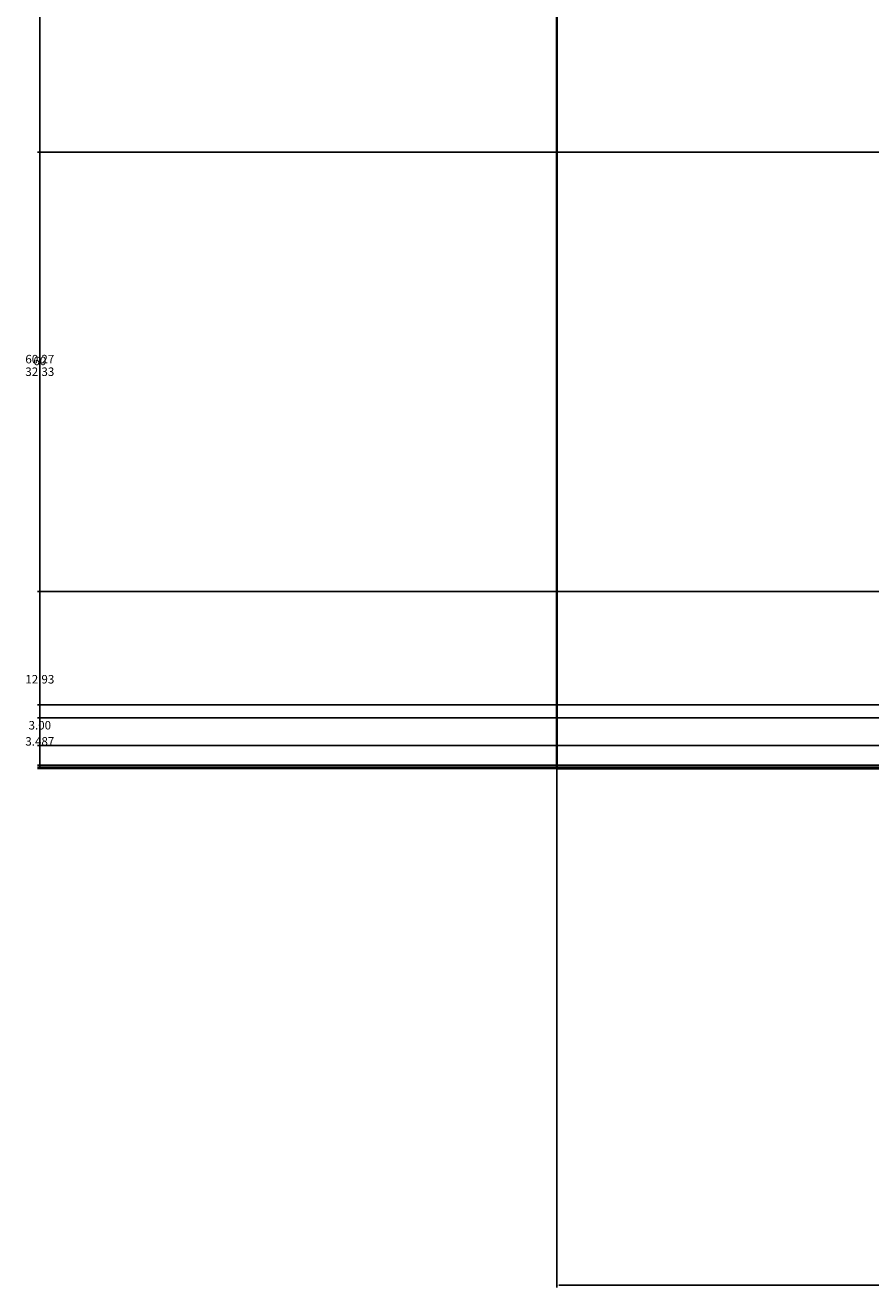
# Model space of a CAD drawing. Units: inches. Extents: x -13 to 809, y 112 to 656.
# Tile 1 of 55: x -13 to 49, y 112 to 205. Entities that reach past the tile are written whole.
import ezdxf

# ---------------------------------------------------------------- set-up
doc = ezdxf.new("R2010")
doc.units = ezdxf.units.IN
doc.header["$MEASUREMENT"] = 0
doc.layers.add('A-ANNO-DIMS', color=2, linetype='Continuous', lineweight=18)
doc.layers.add('A-ELEV', color=7, linetype='Continuous', lineweight=35)
doc.styles.get("Standard").update_dxf_attribs({"font": 'arial.ttf'})
doc.dimstyles.get("Standard").update_dxf_attribs({"dimtxt": 0.625, "dimasz": 0.18, "dimexe": 0.18, "dimexo": 0.0625, "dimgap": 0.09, "dimtad": 0, "dimtih": 1, "dimtoh": 1, "dimdec": 4, "dimzin": 0, "dimdsep": 46, "dimlunit": 4, "dimtxsty": 'Standard', "dimcen": 0.09, "dimadec": 0, "dimazin": 0, "dimtfac": 1, "dimtdec": 4, "dimtofl": 0, "dimtmove": 0, "dimatfit": 3, "dimfxl": 1, "dimtolj": 1, "dimtzin": 0, "dimarcsym": 0})

# ---------------------------------------------------------------- blocks, each defined once
blk = doc.blocks.new('*D11')
at = {"layer": 'A-ANNO-DIMS', "color": 0, "lineweight": -2, "transparency": 16777216}
for p, q in [((95.047, 306.457), (95.047, 112.34)), ((26.081, 150.457), (26.081, 112.34)), ((26.261, 112.52), (59.418, 112.52)), ((94.867, 112.52), (61.71, 112.52))]:
    blk.add_line(p, q, dxfattribs=at)
at = {"layer": 'A-ANNO-DIMS', "color": 0, "transparency": 16777216}
for points in [[(26.261, 112.55), (26.261, 112.49), (26.081, 112.52)], [(94.867, 112.55), (94.867, 112.49), (95.047, 112.52)]]:
    blk.add_solid(points, dxfattribs=at)
at = {"layer": 'Defpoints', "color": 0, "transparency": 16777216}
for p in [(95.047, 306.52), (26.081, 150.52), (95.047, 112.52)]:
    blk.add_point(p, dxfattribs=at)
at = {"layer": 'A-ANNO-DIMS', "color": 0, "transparency": 16777216, "insert": (60.564, 112.52), "char_height": 0.625, "attachment_point": 5}
blk.add_mtext('\\A1;68.97', dxfattribs=at)
blk = doc.blocks.new('*D32')
at = {"layer": 'A-ANNO-DIMS', "color": 0, "lineweight": -2, "transparency": 16777216}
for p, q in [((26.018, 210.52), (-12.099, 210.52)), ((-11.919, 210.34), (-11.919, 180.929)), ((-11.919, 150.7), (-11.919, 180.111)), ((26.018, 150.52), (-12.099, 150.52))]:
    blk.add_line(p, q, dxfattribs=at)
at = {"layer": 'A-ANNO-DIMS', "color": 0, "transparency": 16777216}
for points in [[(-11.949, 210.34), (-11.889, 210.34), (-11.919, 210.52)], [(-11.949, 150.7), (-11.889, 150.7), (-11.919, 150.52)]]:
    blk.add_solid(points, dxfattribs=at)
at = {"layer": 'Defpoints', "color": 0, "transparency": 16777216}
for p in [(-11.919, 210.52), (26.081, 210.52), (26.081, 150.52)]:
    blk.add_point(p, dxfattribs=at)
at = {"layer": 'A-ANNO-DIMS', "color": 0, "transparency": 16777216, "insert": (-11.919, 180.52), "char_height": 0.625, "attachment_point": 5}
blk.add_mtext('\\A1;60', dxfattribs=at)
blk = doc.blocks.new('*D90')
at = {"layer": 'A-ANNO-DIMS', "color": 0, "lineweight": -2, "transparency": 16777216}
for p, q in [((26.081, 210.457), (26.081, 112.34)), ((76.473, 195.828), (76.473, 112.34)), ((26.261, 112.52), (50.132, 112.52)), ((76.293, 112.52), (52.422, 112.52))]:
    blk.add_line(p, q, dxfattribs=at)
at = {"layer": 'A-ANNO-DIMS', "color": 0, "transparency": 16777216}
for points in [[(26.261, 112.55), (26.261, 112.49), (26.081, 112.52)], [(76.293, 112.55), (76.293, 112.49), (76.473, 112.52)]]:
    blk.add_solid(points, dxfattribs=at)
at = {"layer": 'Defpoints', "color": 0, "transparency": 16777216}
for p in [(26.081, 210.52), (76.473, 195.891), (76.473, 112.52)]:
    blk.add_point(p, dxfattribs=at)
at = {"layer": 'A-ANNO-DIMS', "color": 0, "transparency": 16777216, "insert": (51.277, 112.52), "char_height": 0.625, "attachment_point": 5}
blk.add_mtext('\\A1;50.39', dxfattribs=at)
blk = doc.blocks.new('*D91')
at = {"layer": 'A-ANNO-DIMS', "color": 0, "lineweight": -2, "transparency": 16777216}
for p, q in [((76.411, 163.564), (-12.099, 163.564)), ((-11.919, 163.384), (-11.919, 157.508)), ((-11.919, 150.814), (-11.919, 156.69)), ((77.515, 150.634), (-12.099, 150.634))]:
    blk.add_line(p, q, dxfattribs=at)
at = {"layer": 'A-ANNO-DIMS', "color": 0, "transparency": 16777216}
for points in [[(-11.949, 163.384), (-11.889, 163.384), (-11.919, 163.564)], [(-11.949, 150.814), (-11.889, 150.814), (-11.919, 150.634)]]:
    blk.add_solid(points, dxfattribs=at)
at = {"layer": 'Defpoints', "color": 0, "transparency": 16777216}
for p in [(-11.919, 163.564), (76.473, 163.564), (77.577, 150.634)]:
    blk.add_point(p, dxfattribs=at)
at = {"layer": 'A-ANNO-DIMS', "color": 0, "transparency": 16777216, "insert": (-11.919, 157.099), "char_height": 0.625, "attachment_point": 5}
blk.add_mtext('\\A1;12.93', dxfattribs=at)
blk = doc.blocks.new('*D92')
at = {"layer": 'A-ANNO-DIMS', "color": 0, "lineweight": -2, "transparency": 16777216}
for p, q in [((76.411, 195.891), (-12.099, 195.891)), ((-11.919, 195.711), (-11.919, 180.137)), ((-11.919, 163.744), (-11.919, 179.318)), ((76.411, 163.564), (-12.099, 163.564))]:
    blk.add_line(p, q, dxfattribs=at)
at = {"layer": 'A-ANNO-DIMS', "color": 0, "transparency": 16777216}
for points in [[(-11.949, 195.711), (-11.889, 195.711), (-11.919, 195.891)], [(-11.949, 163.744), (-11.889, 163.744), (-11.919, 163.564)]]:
    blk.add_solid(points, dxfattribs=at)
at = {"layer": 'Defpoints', "color": 0, "transparency": 16777216}
for p in [(-11.919, 195.891), (76.473, 195.891), (76.473, 163.564)]:
    blk.add_point(p, dxfattribs=at)
at = {"layer": 'A-ANNO-DIMS', "color": 0, "transparency": 16777216, "insert": (-11.919, 179.727), "char_height": 0.625, "attachment_point": 5}
blk.add_mtext('\\A1;32.33', dxfattribs=at)
blk = doc.blocks.new('*D115')
at = {"layer": 'A-ANNO-DIMS', "color": 0, "lineweight": -2, "transparency": 16777216}
for p, q in [((311.4, 210.785), (-12.099, 210.785)), ((-11.919, 210.605), (-11.919, 181.062)), ((-11.919, 150.7), (-11.919, 180.243)), ((311.637, 150.52), (-12.099, 150.52))]:
    blk.add_line(p, q, dxfattribs=at)
at = {"layer": 'A-ANNO-DIMS', "color": 0, "transparency": 16777216}
for points in [[(-11.949, 210.605), (-11.889, 210.605), (-11.919, 210.785)], [(-11.949, 150.7), (-11.889, 150.7), (-11.919, 150.52)]]:
    blk.add_solid(points, dxfattribs=at)
at = {"layer": 'Defpoints', "color": 0, "transparency": 16777216}
for p in [(-11.919, 210.785), (311.463, 210.785), (311.699, 150.52)]:
    blk.add_point(p, dxfattribs=at)
at = {"layer": 'A-ANNO-DIMS', "color": 0, "transparency": 16777216, "insert": (-11.919, 180.652), "char_height": 0.625, "attachment_point": 5}
blk.add_mtext('\\A1;60.27', dxfattribs=at)
blk = doc.blocks.new('*D117')
at = {"layer": 'A-ANNO-DIMS', "color": 0, "lineweight": -2, "transparency": 16777216}
for p, q in [((260.642, 154.272), (-12.099, 154.272)), ((-11.919, 154.092), (-11.919, 152.938)), ((-11.919, 150.965), (-11.919, 152.119)), ((258.04, 150.785), (-12.099, 150.785))]:
    blk.add_line(p, q, dxfattribs=at)
at = {"layer": 'A-ANNO-DIMS', "color": 0, "transparency": 16777216}
for points in [[(-11.949, 154.092), (-11.889, 154.092), (-11.919, 154.272)], [(-11.949, 150.965), (-11.889, 150.965), (-11.919, 150.785)]]:
    blk.add_solid(points, dxfattribs=at)
at = {"layer": 'Defpoints', "color": 0, "transparency": 16777216}
for p in [(260.705, 154.272), (-11.919, 150.785), (258.102, 150.785)]:
    blk.add_point(p, dxfattribs=at)
at = {"layer": 'A-ANNO-DIMS', "color": 0, "transparency": 16777216, "insert": (-11.919, 152.529), "char_height": 0.625, "attachment_point": 5}
blk.add_mtext('\\A1;3.487', dxfattribs=at)
blk = doc.blocks.new('*D131')
at = {"layer": 'A-ANNO-DIMS', "color": 0, "lineweight": -2, "transparency": 16777216}
for p, q in [((368.876, 155.214), (-12.099, 155.214)), ((-11.919, 155.034), (-11.919, 154.123)), ((-11.919, 152.394), (-11.919, 153.305)), ((365.876, 152.214), (-12.099, 152.214))]:
    blk.add_line(p, q, dxfattribs=at)
at = {"layer": 'A-ANNO-DIMS', "color": 0, "transparency": 16777216}
for points in [[(-11.949, 155.034), (-11.889, 155.034), (-11.919, 155.214)], [(-11.949, 152.394), (-11.889, 152.394), (-11.919, 152.214)]]:
    blk.add_solid(points, dxfattribs=at)
at = {"layer": 'Defpoints', "color": 0, "transparency": 16777216}
for p in [(368.938, 155.214), (-11.919, 152.214), (365.938, 152.214)]:
    blk.add_point(p, dxfattribs=at)
at = {"layer": 'A-ANNO-DIMS', "color": 0, "transparency": 16777216, "insert": (-11.919, 153.714), "char_height": 0.625, "attachment_point": 5}
blk.add_mtext('\\A1;3.00', dxfattribs=at)

msp = doc.modelspace()

# ---------------------------------------------------------------- linework, layer by layer
at = {"layer": 'A-ELEV'}
for p in [(26.0809, 210.5199), (109.5888, 150.5199)]:
    msp.add_line(p, (26.0809, 150.5199), dxfattribs=at)

# ---------------------------------------------------------------- dimensions: what is measured, and where the dimension line sits
at = {"layer": 'A-ANNO-DIMS'}
for base, p1, p2, picture, middle in [((95.0469, 112.5199), (26.0809, 150.5199), (95.0469, 306.5199), '*D11', (60.5639, 112.5199)), ((76.4733, 112.5199), (26.0809, 210.5199), (76.4733, 195.8907), '*D90', (51.2771, 112.5199))]:
    dim = msp.add_linear_dim(base=base, p1=p1, p2=p2, dimstyle='Standard', override={"dimdec": 2, "dimlfac": 1, "dimrnd": 0, "dimzin": 0, "dimdsep": 46, "dimlunit": 2}, dxfattribs=at)
    dim.commit()
    dim.dimension.update_dxf_attribs({"geometry": picture, "text_midpoint": middle})
for base, p1, p2, override, picture, middle in [((-11.91915, 210.78493), (311.6991, 150.51989), (311.46269, 210.78493), {"dimdec": 2, "dimlfac": 1, "dimrnd": 0, "dimzin": 0, "dimdsep": 46, "dimlunit": 2}, '*D115', (-11.91915, 180.65241)), ((-11.9191, 210.5199), (26.0809, 150.5199), (26.0809, 210.5199), {"dimdec": 0, "dimlfac": 1, "dimrnd": 0, "dimzin": 0, "dimdsep": 46, "dimlunit": 2}, '*D32', (-11.9191, 180.5199)), ((-11.9191, 195.8907), (76.4733, 163.5637), (76.4733, 195.8907), {"dimdec": 2, "dimlfac": 1, "dimrnd": 0, "dimzin": 0, "dimdsep": 46, "dimlunit": 2}, '*D92', (-11.9191, 179.7272)), ((-11.9191, 163.5637), (77.5773, 150.6343), (76.4733, 163.5637), {"dimdec": 2, "dimlfac": 1, "dimrnd": 0, "dimzin": 0, "dimdsep": 46, "dimlunit": 2}, '*D91', (-11.9191, 157.099)), ((-11.9191, 152.2141), (368.9383, 155.2141), (365.9383, 152.2141), {"dimdec": 2, "dimlfac": 1, "dimrnd": 0, "dimzin": 0, "dimdsep": 46, "dimlunit": 2}, '*D131', (-11.9191, 153.7141)), ((-11.9191, 150.7849), (260.7048, 154.2723), (258.1022, 150.7849), {"dimdec": 3, "dimlfac": 1, "dimrnd": 0, "dimzin": 0, "dimdsep": 46, "dimlunit": 2}, '*D117', (-11.9191, 152.5286))]:
    dim = msp.add_linear_dim(base=base, p1=p1, p2=p2, angle=90, dimstyle='Standard', override=override, dxfattribs=at)
    dim.commit()
    dim.dimension.update_dxf_attribs({"geometry": picture, "text_midpoint": middle})

doc.saveas('drawing.dxf')
